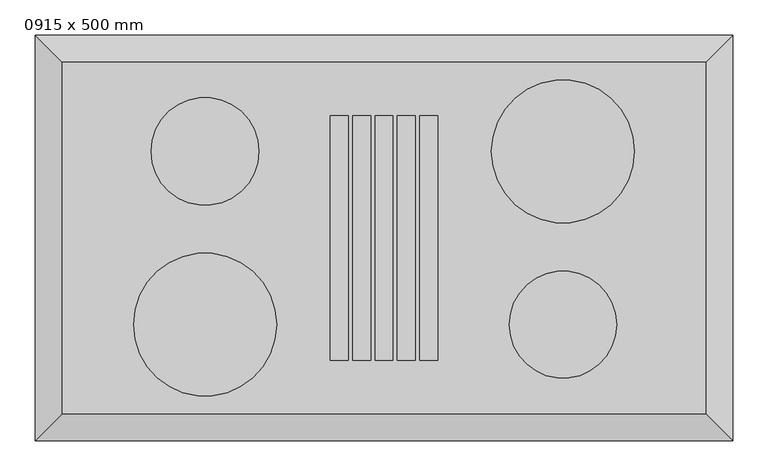
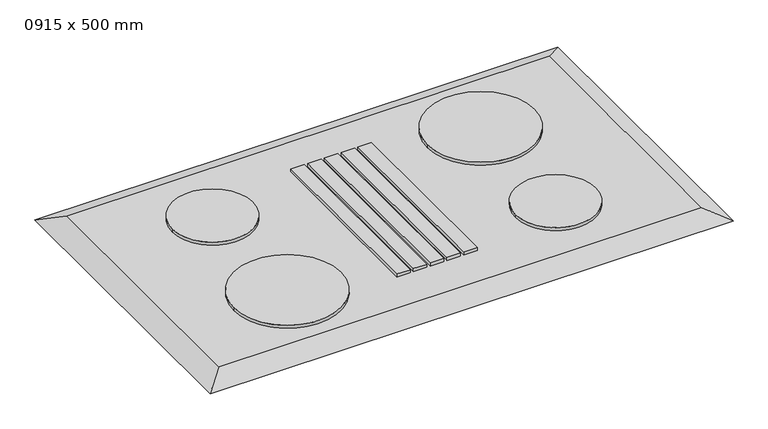
"""IFC4 building model written with IfcOpenShell, lengths in millimetres: proxy geometry, 0915 x 500 mm."""

from ifc_helpers import new_model, si_unit, point, frame, frame_2d, origin, place, context, project, spatial, polyline, circle_curve, trimmed, segment, composite_curve, outline, extrude, faceted_brep, source, transform, mapped, element, save


def proxy_0915_x_500_mm_892363c5(model_context):
    return source(origin(), model_context, "Body", "SolidModel", [
        faceted_brep([(457.5, 250.0, 918.0), (-457.5, 250.0, 918.0), (-457.5, -250.0, 918.0), (457.5, -250.0, 918.0), (495.6, 288.1, 900.0), (495.6, -288.1, 900.0), (-495.6, -288.1, 900.0), (-495.6, 288.1, 900.0)], [[[0, 1, 2, 3]], [[4, 5, 6, 7]], [[4, 7, 1, 0]], [[7, 6, 2, 1]], [[6, 5, 3, 2]], [[5, 4, 0, 3]]]),
        extrude(outline(composite_curve([segment(trimmed(circle_curve(frame_2d((-254.3, 123.0)), 76.5869489), [point((-177.7130511, 123.0))], [point((-330.8869489, 123.0))], False, "CARTESIAN"), True, "CONTINUOUS"), segment(trimmed(circle_curve(frame_2d((-254.3, 123.0)), 76.5869489), [point((-330.8869489, 123.0))], [point((-177.7130511, 123.0))], False, "CARTESIAN"), True, "CONTINUOUS")], self_intersect=False)), frame((0.0, 0.0, 918.0), z_axis=(0.0, 0.0, 1.0), x_axis=(1.0, 0.0, 0.0)), (0.0, 0.0, 1.0), 6.35),
        extrude(outline(composite_curve([segment(trimmed(circle_curve(frame_2d((254.3, 123.0)), 101.6), [point((355.9, 123.0))], [point((152.7, 123.0))], False, "CARTESIAN"), True, "CONTINUOUS"), segment(trimmed(circle_curve(frame_2d((254.3, 123.0)), 101.6), [point((152.7, 123.0))], [point((355.9, 123.0))], False, "CARTESIAN"), True, "CONTINUOUS")], self_intersect=False)), frame((0.0, 0.0, 918.0), z_axis=(0.0, 0.0, 1.0), x_axis=(1.0, 0.0, 0.0)), (0.0, 0.0, 1.0), 6.35),
        extrude(outline(composite_curve([segment(trimmed(circle_curve(frame_2d((254.3, -123.0)), 76.2), [point((330.5, -123.0))], [point((178.1, -123.0))], False, "CARTESIAN"), True, "CONTINUOUS"), segment(trimmed(circle_curve(frame_2d((254.3, -123.0)), 76.2), [point((178.1, -123.0))], [point((330.5, -123.0))], False, "CARTESIAN"), True, "CONTINUOUS")], self_intersect=False)), frame((0.0, 0.0, 918.0), z_axis=(0.0, 0.0, 1.0), x_axis=(1.0, 0.0, 0.0)), (0.0, 0.0, 1.0), 6.35),
        extrude(outline(polyline([(-50.8, 173.8), (-50.8, -173.8), (-76.2, -173.8), (-76.2, 173.8), (-50.8, 173.8)])), frame((0.0, 0.0, 918.0), z_axis=(0.0, 0.0, 1.0), x_axis=(1.0, 0.0, 0.0)), (0.0, 0.0, 1.0), 6.35),
        extrude(outline(polyline([(-19.05, 173.8), (-19.05, -173.8), (-44.45, -173.8), (-44.45, 173.8), (-19.05, 173.8)])), frame((0.0, 0.0, 918.0), z_axis=(0.0, 0.0, 1.0), x_axis=(1.0, 0.0, 0.0)), (0.0, 0.0, 1.0), 6.35),
        extrude(outline(polyline([(12.7, 173.8), (12.7, -173.8), (-12.7, -173.8), (-12.7, 173.8), (12.7, 173.8)])), frame((0.0, 0.0, 918.0), z_axis=(0.0, 0.0, 1.0), x_axis=(1.0, 0.0, 0.0)), (0.0, 0.0, 1.0), 6.35),
        extrude(outline(polyline([(44.45, 173.8), (44.45, -173.8), (19.05, -173.8), (19.05, 173.8), (44.45, 173.8)])), frame((0.0, 0.0, 918.0), z_axis=(0.0, 0.0, 1.0), x_axis=(1.0, 0.0, 0.0)), (0.0, 0.0, 1.0), 6.35),
        extrude(outline(polyline([(76.2, 173.8), (76.2, -173.8), (50.8, -173.8), (50.8, 173.8), (76.2, 173.8)])), frame((0.0, 0.0, 918.0), z_axis=(0.0, 0.0, 1.0), x_axis=(1.0, 0.0, 0.0)), (0.0, 0.0, 1.0), 6.35),
        extrude(outline(composite_curve([segment(trimmed(circle_curve(frame_2d((-254.3, -123.0)), 101.6), [point((-152.7, -123.0))], [point((-355.9, -123.0))], False, "CARTESIAN"), True, "CONTINUOUS"), segment(trimmed(circle_curve(frame_2d((-254.3, -123.0)), 101.6), [point((-355.9, -123.0))], [point((-152.7, -123.0))], False, "CARTESIAN"), True, "CONTINUOUS")], self_intersect=False)), frame((0.0, 0.0, 918.0), z_axis=(0.0, 0.0, 1.0), x_axis=(1.0, 0.0, 0.0)), (0.0, 0.0, 1.0), 6.35),
    ])


if __name__ == "__main__":
    model = new_model("IFC4")
    model_context = context("Model", 3, world=origin())
    ifc_project = project(units=[si_unit("LENGTHUNIT", "METRE", prefix="MILLI")], contexts=[model_context])
    site = spatial("IfcSite", under=ifc_project)
    building = spatial("IfcBuilding", under=site)
    placement = place(None, origin())
    proxy_0915_x_500_mm_shape = proxy_0915_x_500_mm_892363c5(model_context)
    element("IfcBuildingElementProxy", 1, Name="0915 x 500 mm", ObjectType="0915 x 500 mm", at=placement, inside=building, context=model_context, shape_type="MappedRepresentation", body=[
        mapped(proxy_0915_x_500_mm_shape, transform((0.0, 0.0, 0.0), x_axis=(1.0, 0.0, 0.0), y_axis=(0.0, 1.0, 0.0), z_axis=(0.0, 0.0, 1.0))),
    ])
    save(model, "model.ifc")

# Revit data of these elements
# Type "0915 x 500 mm"
#   Profundidad = 500 mm
#   Anchura = 915 mm
#   Máscara [instance default] = yes
#   Quemador = Metal - Cromo
#   Cocina encimera = Metal - Acero, Pulido
#   Default Elevation = 0
# Element 1 (IfcBuildingElementProxy, "0915 x 500 mm")
#   Materials on its faces: "Metal - Cromo", "Metal - Acero, Pulido"
# Materials
#   "Metal - Cromo": class "Metal", colour RGB 17 17 17, transparency 0
#   "Metal - Acero, Pulido": class "Metal", colour RGB 57 57 57, transparency 0
